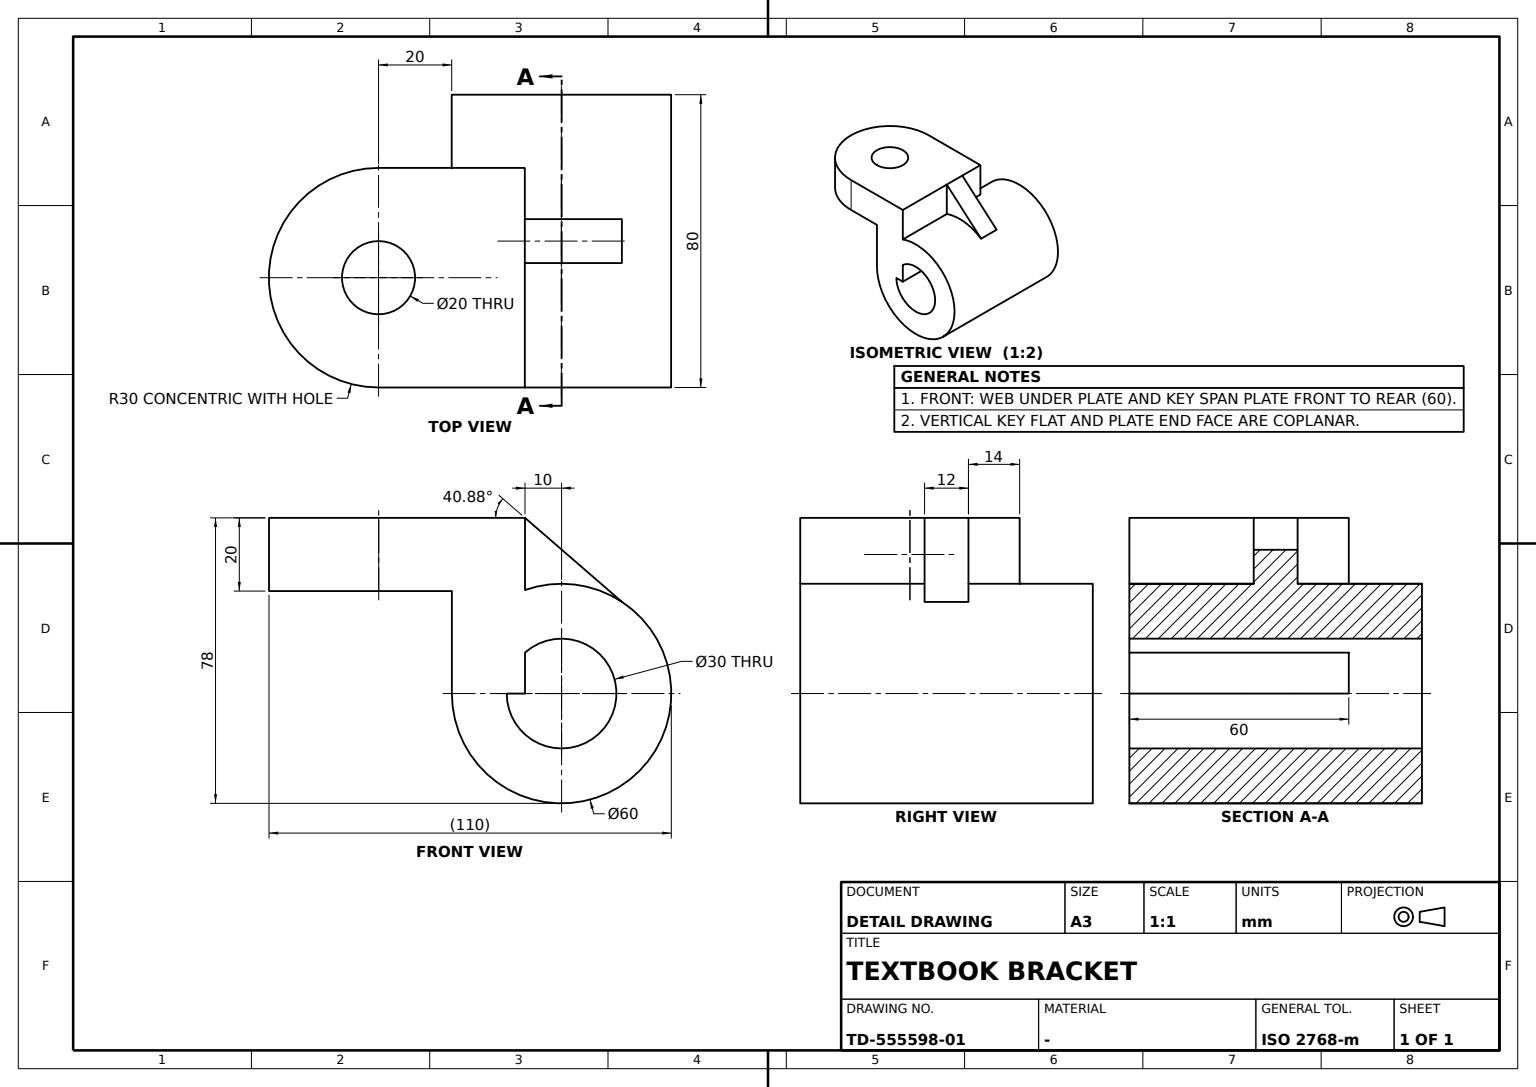
CATIA V5 part; units mm, degrees
sketch "Sketch1" plane through (0, 0, 0) normal (0, 1, 0) x (-1, 0, 0)
  line L0 (0, 0) -> (0, 48)
  line L1 (0, 48) -> (60, 48)
  line L2 (60, 48) -> (60, 0)
  point P0 (60, 0)
  line L3 (60, 0) -> (0, 0)
  dimension "length L2" = 48
  dimension "length L1" = 60
  constraint vertical L0 y-axis
  constraint vertical L2 y-axis
  constraint horizontal L1 x-axis
  constraint horizontal L3 x-axis
  constraint coincidence P0 x-axis
extrude "Pad1" add sketch "Sketch1" along normal mid plane 20
sketch "Sketch3" plane through (0, 0, 48) normal (0, 0, 1) x (1, 0, 0)
  line L0 (-60, 10) -> (-60, -30)
  arc A0 (-60, -30) -> (0, -30) centre (-30, -30) ccw
  point P0 (0, -30)
  line L1 (0, -30) -> (0, 10)
  line L2 (0, 10) -> (-60, 10)
  circle A1 centre (-30, -30) radius 10
  line L3 (-60, 10) -> (0, 10) construction
  dimension "length L2" = 60
  dimension "radius A1" = 10
  dimension "length L1" = 40
  dimension "radius A0" = 30
  constraint vertical L0 y-axis
  constraint coincidence P0 y-axis
  constraint coincidence L2 L3
  constraint tangency A0 L0
  constraint tangency L1 A0
  constraint horizontal L2 x-axis
extrude "Pad2" add sketch "Sketch3" against normal blind 20
sketch "Sketch4" plane through (0, 0, 0) normal (1, 0, 0) x (0, 1, 0)
  circle A0 centre (20, 0) radius 30
  point P0 (20, 0)
  line L0 (-10, 48) -> (-10, 0) construction
  circle A1 centre (20, 0) radius 15
  dimension "radius A0" = 30
  dimension "radius A1" = 15
  constraint coincidence P0 x-axis
  constraint tangency A0 L0
extrude "Pad3" add sketch "Sketch4" against normal blind 80
ref_plane "Plane1" through (-40, 0, 0) normal (1, 0, 0) x (0, 1, 0)
sketch "Sketch5" plane through (-40, 0, 0) normal (1, 0, 0) x (0, 1, 0)
  point P0 (10, 48)
  line L0 (10, 48) -> (36.5369, 25.0306)
  point P1 (36.5369, 25.0306)
  line L1 (10, 48) -> (10, 0) construction
  point P2 (10, 48)
  circle A0 centre (20, 0) radius 30 construction
  constraint coincidence P0 L1
  constraint coincidence P0 P2
  constraint coincidence P1 A0
rib "Stiffener1" sketch "Sketch5" thickness 12 sides both
sketch "Sketch2" plane through (0, 0, 48) normal (0, 0, 1) x (1, 0, 0)
